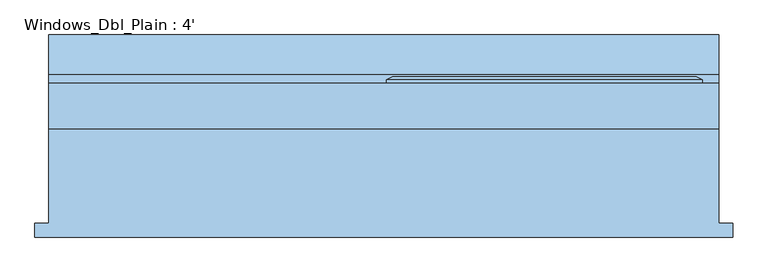
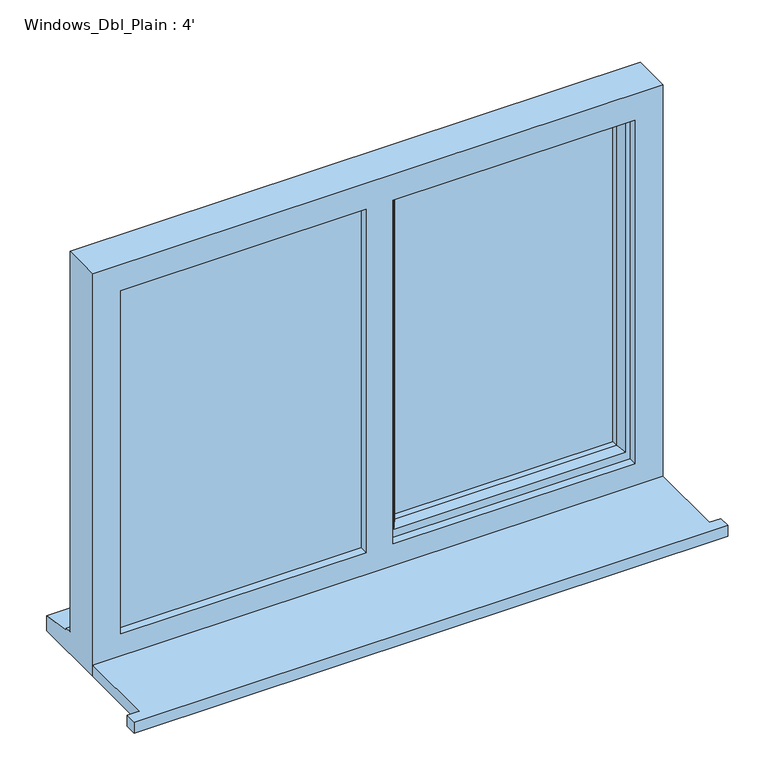
"""IFC4 building model written with IfcOpenShell, lengths in millimetres: window geometry, Windows_Dbl_Plain : 4'."""

from ifc_helpers import new_model, si_unit, frame, origin, place, context, project, spatial, polyline, outline, extrude, faceted_brep, source, transform, mapped, element, save


def windows_dbl_plain_4_ad201dc9(model_context):
    return source(origin(), model_context, "Body", "SolidModel", [
        extrude(outline(polyline([(-919.6, -168.9434322), (-919.6, -143.9434322), (-894.6, -143.9434322), (-894.6, 27.8565678), (324.6, 27.8565678), (324.6, -143.9434322), (349.6, -143.9434322), (349.6, -168.9434322), (-919.6, -168.9434322)])), frame((0.0, 0.0, 1200.0), z_axis=(0.0, 0.0, 1.0), x_axis=(1.0, 0.0, 0.0)), (0.0, 0.0, 1.0), 25.0),
        faceted_brep([(-280.0, 110.8565678, 2080.0), (-280.0, 116.6300705, 2080.0), (-280.0, 116.6300705, 1253.0), (-280.0, 110.8565678, 1253.0), (-270.0, 45.8565678, 2070.0), (-270.0, 110.8565678, 2070.0), (-270.0, 110.8565678, 1263.0), (-270.0, 45.8565678, 1263.0), (-230.0, 60.3494677, 2030.0), (-240.1480377, 45.8565678, 2040.1480377), (-240.1480377, 45.8565678, 1292.8519623), (-230.0, 60.3494677, 1303.0), (-230.0, 74.8565678, 2030.0), (-230.0, 74.8565678, 1303.0), (-240.0, 98.8565678, 2040.0), (-240.0, 74.8565678, 2040.0), (-240.0, 74.8565678, 1293.0), (-240.0, 98.8565678, 1293.0), (-230.0, 116.6300705, 2030.0), (-230.0, 98.8565678, 2030.0), (-230.0, 98.8565678, 1303.0), (-230.0, 116.6300705, 1303.0), (-247.4457548, 122.4035732, 2047.4457548), (-247.4457548, 122.4035732, 1285.5542452), (-269.2153903, 122.4035732, 2069.2153903), (-269.2153903, 122.4035732, 1263.7846097), (294.6, 116.6300705, 1253.0), (294.6, 110.8565678, 1253.0), (284.6, 110.8565678, 1263.0), (284.6, 45.8565678, 1263.0), (254.7480377, 45.8565678, 1292.8519623), (244.6, 60.3494677, 1303.0), (244.6, 74.8565678, 1303.0), (254.6, 74.8565678, 1293.0), (254.6, 98.8565678, 1293.0), (244.6, 98.8565678, 1303.0), (244.6, 116.6300705, 1303.0), (262.0457548, 122.4035732, 1285.5542452), (283.8153903, 122.4035732, 1263.7846097), (294.6, 116.6300705, 2080.0), (294.6, 110.8565678, 2080.0), (284.6, 110.8565678, 2070.0), (284.6, 45.8565678, 2070.0), (254.7480377, 45.8565678, 2040.1480377), (244.6, 60.3494677, 2030.0), (244.6, 74.8565678, 2030.0), (254.6, 74.8565678, 2040.0), (254.6, 98.8565678, 2040.0), (244.6, 98.8565678, 2030.0), (244.6, 116.6300705, 2030.0), (262.0457548, 122.4035732, 2047.4457548), (283.8153903, 122.4035732, 2069.2153903)], [[[0, 1, 2, 3]], [[4, 5, 6, 7]], [[8, 9, 10, 11]], [[12, 8, 11, 13]], [[14, 15, 16, 17]], [[18, 19, 20, 21]], [[22, 18, 21, 23]], [[1, 24, 25, 2]], [[3, 2, 26, 27]], [[7, 6, 28, 29]], [[11, 10, 30, 31]], [[13, 11, 31, 32]], [[17, 16, 33, 34]], [[21, 20, 35, 36]], [[23, 21, 36, 37]], [[2, 25, 38, 26]], [[27, 26, 39, 40]], [[29, 28, 41, 42]], [[31, 30, 43, 44]], [[32, 31, 44, 45]], [[34, 33, 46, 47]], [[36, 35, 48, 49]], [[37, 36, 49, 50]], [[26, 38, 51, 39]], [[40, 39, 1, 0]], [[3, 27, 40, 0], [5, 41, 28, 6]], [[42, 41, 5, 4]], [[7, 29, 42, 4], [9, 43, 30, 10]], [[44, 43, 9, 8]], [[45, 44, 8, 12]], [[15, 46, 33, 16], [13, 32, 45, 12]], [[47, 46, 15, 14]], [[17, 34, 47, 14], [19, 48, 35, 20]], [[49, 48, 19, 18]], [[50, 49, 18, 22]], [[24, 51, 38, 25], [23, 37, 50, 22]], [[39, 51, 24, 1]]]),
        extrude(outline(polyline([(2050.0, -310.0), (2070.0, -310.0), (2070.0, -854.6), (1263.0, -854.6), (1263.0, -310.0), (1283.0, -310.0), (1283.0, -834.6), (2050.0, -834.6), (2050.0, -310.0)])), frame((0.0, 69.8565678, 0.0), z_axis=(0.0, 1.0, 0.0), x_axis=(0.0, 0.0, 1.0)), (0.0, 0.0, 1.0), 41.0),
        faceted_brep([(324.6, 27.8565678, 2110.0), (-894.6, 27.8565678, 2110.0), (-894.6, 27.8565678, 1200.0), (324.6, 27.8565678, 1200.0), (264.6, 27.8565678, 2050.0), (264.6, 27.8565678, 1275.0), (-252.0, 27.8565678, 1275.0), (-252.0, 27.8565678, 2050.0), (-310.0, 27.8565678, 2050.0), (-310.0, 27.8565678, 1275.0), (-834.6, 27.8565678, 1275.0), (-834.6, 27.8565678, 2050.0), (-894.6, 110.8565678, 2110.0), (-894.6, 110.8565678, 1251.0), (-894.6, 125.8565678, 1249.68767), (-894.6, 125.8565678, 1244.7449676), (-894.6, 198.3565678, 1233.8088847), (-894.6, 198.3565678, 1200.0), (324.6, 110.8565678, 2110.0), (324.6, 110.8565678, 1251.0), (-854.6, 110.8565678, 2070.0), (-854.6, 110.8565678, 1263.0), (-310.0, 110.8565678, 1263.0), (-310.0, 110.8565678, 2070.0), (-270.0, 110.8565678, 2070.0), (-270.0, 110.8565678, 1263.0), (284.6, 110.8565678, 1263.0), (284.6, 110.8565678, 2070.0), (-854.6, 45.8565678, 2070.0), (-854.6, 45.8565678, 1263.0), (-300.0, 45.8565678, 2070.0), (-300.0, 45.8565678, 1263.0), (-310.0, 45.8565678, 2050.0), (-834.6, 45.8565678, 2050.0), (-834.6, 45.8565678, 1275.0), (-310.0, 45.8565678, 1275.0), (-270.0, 45.8565678, 2070.0), (284.6, 45.8565678, 2070.0), (284.6, 45.8565678, 1263.0), (-270.0, 45.8565678, 1263.0), (264.6, 45.8565678, 2050.0), (-252.0, 45.8565678, 2050.0), (-252.0, 45.8565678, 1275.0), (264.6, 45.8565678, 1275.0), (-310.0, 69.8565678, 2070.0), (-300.0, 69.8565678, 2070.0), (324.6, 198.3565678, 1200.0), (324.6, 198.3565678, 1233.8088847), (324.6, 125.8565678, 1244.7449676), (324.6, 125.8565678, 1249.68767), (-300.0, 69.8565678, 1263.0), (-310.0, 69.8565678, 1263.0)], [[[0, 1, 2, 3], [4, 5, 6, 7], [8, 9, 10, 11]], [[2, 1, 12, 13, 14, 15, 16, 17]], [[13, 12, 18, 19], [20, 21, 22, 23], [24, 25, 26, 27]], [[21, 20, 28, 29]], [[28, 30, 31, 29], [32, 33, 34, 35]], [[36, 37, 38, 39], [40, 41, 42, 43]], [[33, 11, 10, 34]], [[1, 0, 18, 12]], [[28, 20, 23, 44, 45, 30]], [[27, 37, 36, 24]], [[11, 33, 32, 8]], [[40, 4, 7, 41]], [[19, 18, 0, 3, 46, 47, 48, 49]], [[27, 26, 38, 37]], [[4, 40, 43, 5]], [[45, 50, 31, 30]], [[50, 45, 44, 51]], [[51, 44, 23, 22]], [[25, 24, 36, 39]], [[41, 7, 6, 42]], [[8, 32, 35, 9]], [[46, 3, 2, 17]], [[47, 46, 17, 16]], [[48, 47, 16, 15]], [[49, 48, 15, 14]], [[19, 49, 14, 13]], [[22, 21, 29, 31, 50, 51]], [[26, 25, 39, 38]], [[6, 5, 43, 42]], [[35, 34, 10, 9]]]),
        extrude(outline(polyline([(-854.6, 69.8565678), (-300.0, 69.8565678), (-300.0, 45.8565678), (-854.6, 45.8565678), (-854.6, 69.8565678)])), frame((0.0, 0.0, 1263.0), z_axis=(0.0, 0.0, 1.0), x_axis=(1.0, 0.0, 0.0)), (0.0, 0.0, 1.0), 807.0),
        extrude(outline(polyline([(254.6, 74.8565678), (-240.0, 74.8565678), (-240.0, 98.8565678), (254.6, 98.8565678), (254.6, 74.8565678)])), frame((0.0, 0.0, 1293.0), z_axis=(0.0, 0.0, 1.0), x_axis=(1.0, 0.0, 0.0)), (0.0, 0.0, 1.0), 747.0),
    ])


if __name__ == "__main__":
    model = new_model("IFC4")
    model_context = context("Model", 3, world=origin())
    ifc_project = project(units=[si_unit("LENGTHUNIT", "METRE", prefix="MILLI")], contexts=[model_context])
    site = spatial("IfcSite", under=ifc_project)
    building = spatial("IfcBuilding", under=site)
    placement = place(None, origin())
    windows_dbl_plain_4_shape = windows_dbl_plain_4_ad201dc9(model_context)
    element("IfcWindow", 1, ObjectType="Windows_Dbl_Plain : 4'", at=placement, inside=building, context=model_context, shape_type="MappedRepresentation", body=[
        mapped(windows_dbl_plain_4_shape, transform((0.0, 0.0, 0.0), x_axis=(1.0, 0.0, 0.0), y_axis=(0.0, 1.0, 0.0), z_axis=(0.0, 0.0, 1.0))),
    ])
    save(model, "model.ifc")

# Revit data of these elements
# Type "Windows_Dbl_Plain : 4'"
#   Type Mark = "56"
#   Operation = "DoublePanelVertical"
#   Construction Type Id = "GSP4R"
#   Manufacturer = "Revit"
#   Keynote = "L10"
#   Analytic Construction = "1/8 in Pilkington single glazing"
#   Wrap Layers (Ext) from Ext = 0.336286 ft
#   Wrap Layers (Int) from Ext = 0.582349 ft
#   Window Board Projection = 0.082021 ft
#   Window Board Extension = 0.082021 ft
#   Visual Light Transmittance = 0.9
#   Solar Heat Gain Coefficient = 0.78
#   Rough Width = 4.0 ft
#   Rough Height = 2.985564 ft
#   Height = 2.985564 ft
#   Width = 4.0 ft
#   Heat Transfer Coefficient (U) = 3.6886 W/(m²·K)
#   Glazing Thickness = 0.07874 ft
#   FrameOffset - External = 0.164042 ft
#   Frame Depth = 0.213255 ft
#   Default Head Height = 6.922572 ft
#   Cill Depth = 0.287073 ft
#   Cavity Closer Width = 0.164042 ft
#   Cavity Closer Offset from Ext = 0.336286 ft
#   Cavity Closer Depth = 0.278871 ft
#   Vis - Cavity Closers = yes
#   Define Thermal Properties by = 1
#   Material Trim = Window Frame
#   Material Glass = Glass
#   Material Frame = Window Frame
#   Wall Closure = (empty or 0)
# Element 1 (IfcWindow, "Windows_Dbl_Plain : 4'")
#   Materials on its faces: "Window Frame", "Glass"
# Materials
#   "Window Frame": colour RGB 249 249 249, transparency 0, Keynote = "L10", Cost = 0
#   "Glass": class "Glass", colour RGB 0 128 192, transparency 0.9, Description = "Soda Lime Glass", Cost = 0
